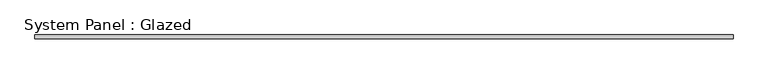
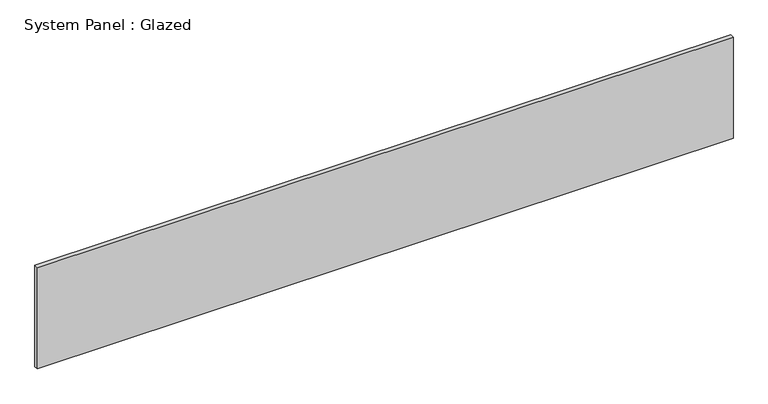
"""IFC4 building model written with IfcOpenShell, lengths in millimetres: plate geometry, System Panel : Glazed."""

from ifc_helpers import new_model, si_unit, origin, origin_with_axes, place, context, project, spatial, polyline, outline, extrude, source, transform, mapped, element, save


def system_panel_glazed_bff90f26(model_context):
    return source(origin(), model_context, "Body", "SweptSolid", [
        extrude(outline(polyline([(2182.1604725, 19.05), (-2182.1604725, 19.05), (-2182.1604725, 44.45), (2182.1604725, 44.45), (2182.1604725, 19.05)])), origin_with_axes(), (0.0, 0.0, 1.0), 670.8053209),
    ])


if __name__ == "__main__":
    model = new_model("IFC4")
    model_context = context("Model", 3, world=origin())
    ifc_project = project(units=[si_unit("LENGTHUNIT", "METRE", prefix="MILLI")], contexts=[model_context])
    site = spatial("IfcSite", under=ifc_project)
    building = spatial("IfcBuilding", under=site)
    placement = place(None, origin())
    system_panel_glazed_shape = system_panel_glazed_bff90f26(model_context)
    element("IfcPlate", 1, ObjectType="System Panel : Glazed", at=placement, inside=building, context=model_context, shape_type="MappedRepresentation", body=[
        mapped(system_panel_glazed_shape, transform((0.0, 0.0, 0.0), x_axis=(1.0, 0.0, 0.0), y_axis=(0.0, 1.0, 0.0), z_axis=(0.0, 0.0, 1.0))),
    ])
    save(model, "model.ifc")

# Revit data of these elements
# Type "System Panel : Glazed"
#   Construction Type Id = "GSP4R"
#   Analytic Construction = "1/8 in Pilkington single glazing"
#   Visual Light Transmittance = 0.9
#   Solar Heat Gain Coefficient = 0.86
#   Heat Transfer Coefficient (U) = 1.18115 BTU/(h·ft²·°F)
#   Define Thermal Properties by = 1
# Element 1 (IfcPlate, "System Panel : Glazed")
#   Materials on its faces: "Glass"
# Materials
#   "Glass": class "Glass", colour RGB 0 128 192, transparency 0.75, Description = "Soda Lime Glass", Cost = 0
